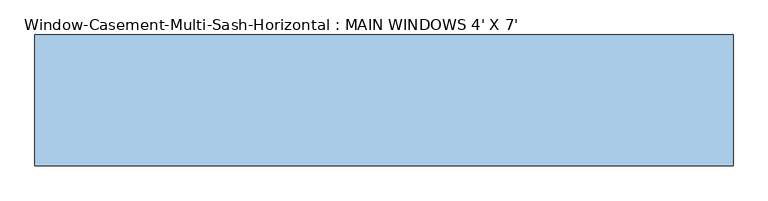
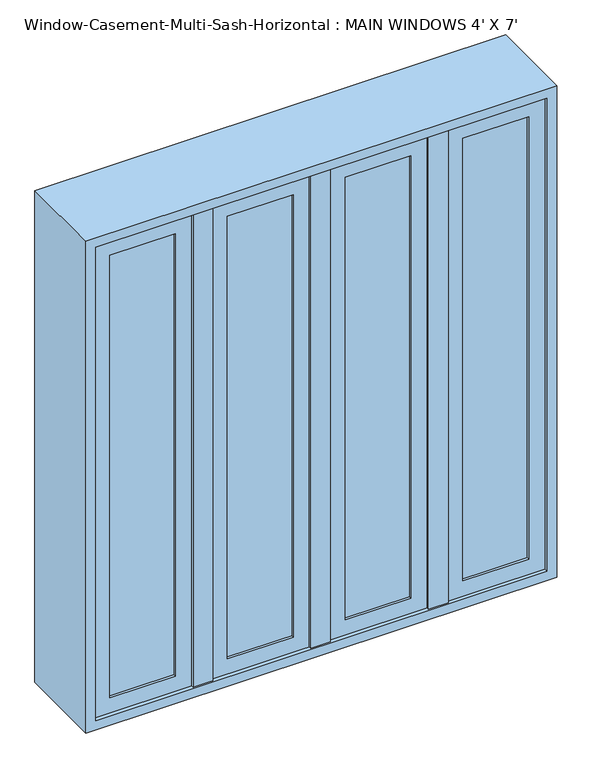
"""IFC4 building model written with IfcOpenShell, lengths in millimetres: window geometry, Window-Casement-Multi-Sash-Horizontal : MAIN WINDOWS 4' X 7'."""

from ifc_helpers import new_model, si_unit, frame, origin, place, context, project, spatial, polyline, outline, extrude, faceted_brep, source, transform, mapped, element, save


def window_casement_multi_sash_horizontal_main_windows_4_x_7_c0e1ebbb(model_context):
    return source(origin(), model_context, "Body", "SolidModel", [
        extrude(outline(polyline([(2235.2, 584.2), (2235.2, 330.2), (939.8, 330.2), (939.8, 584.2), (2235.2, 584.2)]), holes=[polyline([(2193.3296875, 372.0703125), (2193.3296875, 542.3296875), (981.6703125, 542.3296875), (981.6703125, 372.0703125), (2193.3296875, 372.0703125)])]), frame((0.0, -104.775, 0.0), z_axis=(0.0, 1.0, 0.0), x_axis=(0.0, 0.0, 1.0)), (0.0, 0.0, 1.0), 31.75),
        extrude(outline(polyline([(2235.2, -330.2), (2235.2, -584.2), (939.8, -584.2), (939.8, -330.2), (2235.2, -330.2)]), holes=[polyline([(2193.3296875, -542.3296875), (2193.3296875, -372.0703125), (981.6703125, -372.0703125), (981.6703125, -542.3296875), (2193.3296875, -542.3296875)])]), frame((0.0, -104.775, 0.0), z_axis=(0.0, 1.0, 0.0), x_axis=(0.0, 0.0, 1.0)), (0.0, 0.0, 1.0), 31.75),
        extrude(outline(polyline([(-372.0703125, -98.425), (-542.3296875, -98.425), (-542.3296875, -92.075), (-372.0703125, -92.075), (-372.0703125, -98.425)])), frame((0.0, 0.0, 981.6703125), z_axis=(0.0, 0.0, 1.0), x_axis=(1.0, 0.0, 0.0)), (0.0, 0.0, 1.0), 1211.659375),
        extrude(outline(polyline([(-372.0703125, -85.725), (-542.3296875, -85.725), (-542.3296875, -79.375), (-372.0703125, -79.375), (-372.0703125, -85.725)])), frame((0.0, 0.0, 981.6703125), z_axis=(0.0, 0.0, 1.0), x_axis=(1.0, 0.0, 0.0)), (0.0, 0.0, 1.0), 1211.659375),
        extrude(outline(polyline([(542.3296875, -98.425), (372.0703125, -98.425), (372.0703125, -92.075), (542.3296875, -92.075), (542.3296875, -98.425)])), frame((0.0, 0.0, 981.6703125), z_axis=(0.0, 0.0, 1.0), x_axis=(1.0, 0.0, 0.0)), (0.0, 0.0, 1.0), 1211.659375),
        extrude(outline(polyline([(542.3296875, -85.725), (372.0703125, -85.725), (372.0703125, -79.375), (542.3296875, -79.375), (542.3296875, -85.725)])), frame((0.0, 0.0, 981.6703125), z_axis=(0.0, 0.0, 1.0), x_axis=(1.0, 0.0, 0.0)), (0.0, 0.0, 1.0), 1211.659375),
        extrude(outline(polyline([(-67.2703125, -98.425), (-237.5296875, -98.425), (-237.5296875, -92.075), (-67.2703125, -92.075), (-67.2703125, -98.425)])), frame((0.0, 0.0, 981.6703125), z_axis=(0.0, 0.0, 1.0), x_axis=(1.0, 0.0, 0.0)), (0.0, 0.0, 1.0), 1211.659375),
        extrude(outline(polyline([(-67.2703125, -85.725), (-237.5296875, -85.725), (-237.5296875, -79.375), (-67.2703125, -79.375), (-67.2703125, -85.725)])), frame((0.0, 0.0, 981.6703125), z_axis=(0.0, 0.0, 1.0), x_axis=(1.0, 0.0, 0.0)), (0.0, 0.0, 1.0), 1211.659375),
        extrude(outline(polyline([(237.5296875, -98.425), (67.2703125, -98.425), (67.2703125, -92.075), (237.5296875, -92.075), (237.5296875, -98.425)])), frame((0.0, 0.0, 981.6703125), z_axis=(0.0, 0.0, 1.0), x_axis=(1.0, 0.0, 0.0)), (0.0, 0.0, 1.0), 1211.659375),
        extrude(outline(polyline([(237.5296875, -85.725), (67.2703125, -85.725), (67.2703125, -79.375), (237.5296875, -79.375), (237.5296875, -85.725)])), frame((0.0, 0.0, 981.6703125), z_axis=(0.0, 0.0, 1.0), x_axis=(1.0, 0.0, 0.0)), (0.0, 0.0, 1.0), 1211.659375),
        faceted_brep([(-330.2, -73.025, 2235.2), (-330.2, -111.125, 2235.2), (-279.4, -111.125, 2235.2), (-279.4, -73.025, 2235.2), (-25.4, -73.025, 2235.2), (-25.4, -111.125, 2235.2), (25.4, -111.125, 2235.2), (25.4, -73.025, 2235.2), (279.4, -73.025, 2235.2), (279.4, -111.125, 2235.2), (330.2, -111.125, 2235.2), (330.2, -73.025, 2235.2), (584.2, -73.025, 2235.2), (584.2, -114.3, 2235.2), (-584.2, -114.3, 2235.2), (-584.2, -73.025, 2235.2), (-574.0796875, -22.225, 2225.0796875), (-340.3203125, -22.225, 2225.0796875), (-340.3203125, -73.025, 2225.0796875), (-574.0796875, -73.025, 2225.0796875), (574.0796875, -73.025, 2225.0796875), (340.3203125, -73.025, 2225.0796875), (340.3203125, -22.225, 2225.0796875), (574.0796875, -22.225, 2225.0796875), (-269.2796875, -73.025, 2225.0796875), (-269.2796875, -22.225, 2225.0796875), (-35.5203125, -22.225, 2225.0796875), (-35.5203125, -73.025, 2225.0796875), (35.5203125, -73.025, 2225.0796875), (35.5203125, -22.225, 2225.0796875), (269.2796875, -22.225, 2225.0796875), (269.2796875, -73.025, 2225.0796875), (-584.2, 114.3, 2235.2), (584.2, 114.3, 2235.2), (584.2, -22.225, 2235.2), (-584.2, -22.225, 2235.2), (-609.6, -114.3, 2260.6), (609.6, -114.3, 2260.6), (609.6, 114.3, 2260.6), (-609.6, 114.3, 2260.6), (584.2, -73.025, 939.8), (584.2, -114.3, 939.8), (574.0796875, -22.225, 949.9203125), (574.0796875, -73.025, 949.9203125), (584.2, 114.3, 939.8), (584.2, -22.225, 939.8), (609.6, -114.3, 914.4), (609.6, 114.3, 914.4), (330.2, -73.025, 939.8), (330.2, -111.125, 939.8), (279.4, -111.125, 939.8), (279.4, -73.025, 939.8), (25.4, -73.025, 939.8), (25.4, -111.125, 939.8), (-25.4, -111.125, 939.8), (-25.4, -73.025, 939.8), (-279.4, -73.025, 939.8), (-279.4, -111.125, 939.8), (-330.2, -111.125, 939.8), (-330.2, -73.025, 939.8), (-584.2, -73.025, 939.8), (-584.2, -114.3, 939.8), (340.3203125, -22.225, 949.9203125), (340.3203125, -73.025, 949.9203125), (-574.0796875, -73.025, 949.9203125), (-340.3203125, -73.025, 949.9203125), (-340.3203125, -22.225, 949.9203125), (-574.0796875, -22.225, 949.9203125), (-35.5203125, -73.025, 949.9203125), (-35.5203125, -22.225, 949.9203125), (-269.2796875, -22.225, 949.9203125), (-269.2796875, -73.025, 949.9203125), (269.2796875, -73.025, 949.9203125), (269.2796875, -22.225, 949.9203125), (35.5203125, -22.225, 949.9203125), (35.5203125, -73.025, 949.9203125), (-584.2, 114.3, 939.8), (-584.2, -22.225, 939.8), (-609.6, -114.3, 914.4), (-609.6, 114.3, 914.4)], [[[0, 1, 2, 3, 4, 5, 6, 7, 8, 9, 10, 11, 12, 13, 14, 15]], [[16, 17, 18, 19]], [[20, 21, 22, 23]], [[24, 25, 26, 27]], [[28, 29, 30, 31]], [[32, 33, 34, 35]], [[36, 37, 38, 39]], [[12, 40, 41, 13]], [[23, 42, 43, 20]], [[33, 44, 45, 34]], [[37, 46, 47, 38]], [[48, 49, 50, 51, 52, 53, 54, 55, 56, 57, 58, 59, 60, 61, 41, 40]], [[42, 62, 63, 43]], [[64, 65, 66, 67]], [[68, 69, 70, 71]], [[72, 73, 74, 75]], [[44, 76, 77, 45]], [[46, 78, 79, 47]], [[14, 61, 60, 15]], [[12, 11, 48, 40], [20, 43, 63, 21]], [[8, 7, 52, 51], [75, 28, 31, 72]], [[4, 3, 56, 55], [71, 24, 27, 68]], [[60, 59, 0, 15], [64, 19, 18, 65]], [[19, 64, 67, 16]], [[45, 77, 35, 34], [23, 22, 62, 42], [16, 67, 66, 17], [25, 70, 69, 26], [29, 74, 73, 30]], [[35, 77, 76, 32]], [[38, 47, 79, 39], [32, 76, 44, 33]], [[39, 79, 78, 36]], [[36, 78, 46, 37], [13, 41, 61, 14]], [[18, 17, 66, 65]], [[71, 70, 25, 24]], [[57, 56, 3, 2]], [[2, 1, 58, 57]], [[1, 0, 59, 58]], [[27, 26, 69, 68]], [[75, 74, 29, 28]], [[53, 52, 7, 6]], [[6, 5, 54, 53]], [[5, 4, 55, 54]], [[10, 9, 50, 49]], [[9, 8, 51, 50]], [[31, 30, 73, 72]], [[63, 62, 22, 21]], [[49, 48, 11, 10]]]),
        extrude(outline(polyline([(2235.2, 279.4), (2235.2, 25.4), (939.8, 25.4), (939.8, 279.4), (2235.2, 279.4)]), holes=[polyline([(2193.3296875, 67.2703125), (2193.3296875, 237.5296875), (981.6703125, 237.5296875), (981.6703125, 67.2703125), (2193.3296875, 67.2703125)])]), frame((0.0, -104.775, 0.0), z_axis=(0.0, 1.0, 0.0), x_axis=(0.0, 0.0, 1.0)), (0.0, 0.0, 1.0), 31.75),
        extrude(outline(polyline([(2235.2, -25.4), (2235.2, -279.4), (939.8, -279.4), (939.8, -25.4), (2235.2, -25.4)]), holes=[polyline([(2193.3296875, -237.5296875), (2193.3296875, -67.2703125), (981.6703125, -67.2703125), (981.6703125, -237.5296875), (2193.3296875, -237.5296875)])]), frame((0.0, -104.775, 0.0), z_axis=(0.0, 1.0, 0.0), x_axis=(0.0, 0.0, 1.0)), (0.0, 0.0, 1.0), 31.75),
    ])


if __name__ == "__main__":
    model = new_model("IFC4")
    model_context = context("Model", 3, world=origin())
    ifc_project = project(units=[si_unit("LENGTHUNIT", "METRE", prefix="MILLI")], contexts=[model_context])
    site = spatial("IfcSite", under=ifc_project)
    building = spatial("IfcBuilding", under=site)
    placement = place(None, origin())
    window_casement_multi_sash_horizontal_main_windows_4_x_7_shape = window_casement_multi_sash_horizontal_main_windows_4_x_7_c0e1ebbb(model_context)
    element("IfcWindow", 1, ObjectType="Window-Casement-Multi-Sash-Horizontal : MAIN WINDOWS 4' X 7'", at=placement, inside=building, context=model_context, shape_type="MappedRepresentation", body=[
        mapped(window_casement_multi_sash_horizontal_main_windows_4_x_7_shape, transform((0.0, 0.0, 0.0), x_axis=(1.0, 0.0, 0.0), y_axis=(0.0, 1.0, 0.0), z_axis=(0.0, 0.0, 1.0))),
    ])
    save(model, "model.ifc")

# Revit data of these elements
# Type "Window-Casement-Multi-Sash-Horizontal : MAIN WINDOWS 4' X 7'"
#   Type Mark = "21"
#   Fire Rating = "0.5h"
#   Assembly Code = "B2020100"
#   Analytic Construction = "Double glazing - domestic"
#   Window Inset [instance default] = 0' - 0 5/8"
#   Wall Thickness [instance default] = 0' - 6"
#   Visual Light Transmittance = 0.81
#   Thermal Resistance (R) = 1.8146 (h·ft²·°F)/BTU
#   Solar Heat Gain Coefficient = 0.76
#   Rough Width = 4' - 0 1/2"
#   Rough Height = 4' - 5 1/2"
#   Open Window Width = 1' - 0"
#   Heat Transfer Coefficient (U) = 0.5511 BTU/(h·ft²·°F)
#   Height = 4' - 5"
#   Frame Gap 3 [instance default] = 0' - 1 83/128"
#   Frame Gap 2 [instance default] = 0' - 0 5/8"
#   Frame Gap 1 = 0' - 1 51/128"
#   Default Sill Height = 3' - 0"
#   Width = 4' - 0"
#   Frame Material = Metal - Aluminum
#   Glass Panel Material = Glass
#   Wall Closure = (empty or 0)
# Element 1 (IfcWindow, "Window-Casement-Multi-Sash-Horizontal : MAIN WINDOWS 4' X 7'")
#   Wall Thickness = 0' - 9"
#   Materials on its faces: "Metal - Aluminum", "Glass"
# Materials
#   "Metal - Aluminum": class "Metal", colour RGB 247 247 247, transparency 0
#   "Glass": class "Glass", colour RGB 0 128 192, transparency 0.75, Description = "Soda Lime Glass", Cost = 0
